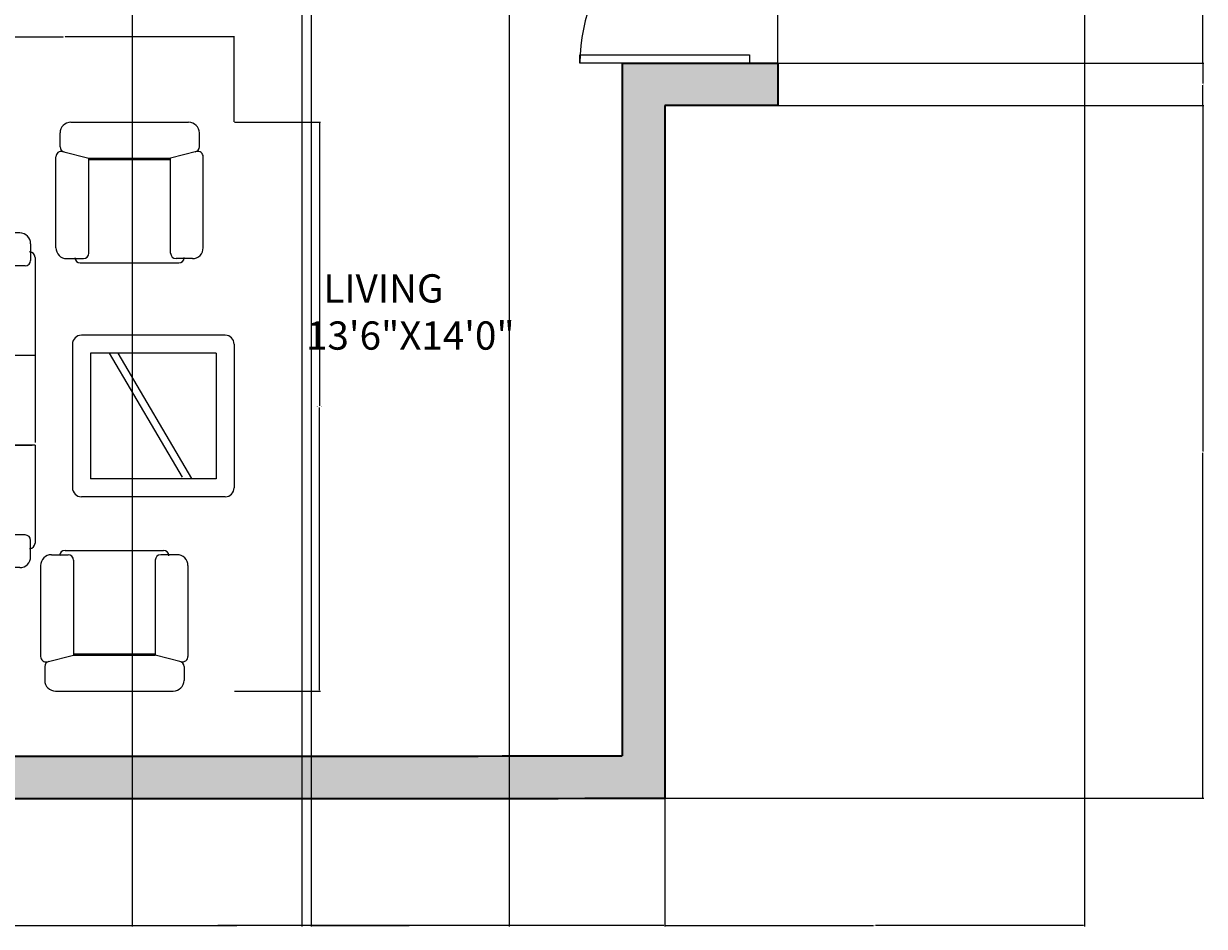
# Model space of a CAD drawing. Units: inches. Extents: x 1044 to 1567, y 918 to 1417.
# Tile 3 of 4: x 1316 to 1567, y 918 to 1110. Entities that reach past the tile are written whole.
import ezdxf

# ---------------------------------------------------------------- set-up
doc = ezdxf.new("R2010")
doc.units = ezdxf.units.IN
for name, color, linetype, lineweight in [('A-ANNO-DIMS', 2, 'Continuous', 18), ('A-AREA-IDEN', 7, 'Continuous', 18), ('A-FLOR', 7, 'Continuous', 13), ('A-FURN', 8, 'Continuous', 18), ('A-WALL', 7, 'Continuous', 35), ('A-WALL-PATT', 252, 'Continuous', 13), ('door', 4, 'Continuous', 18)]:
    doc.layers.add(name, color=color, linetype=linetype, lineweight=lineweight)
doc.styles.get("Standard").update_dxf_attribs({"font": 'arial.ttf'})
doc.dimstyles.get("Standard").update_dxf_attribs({"dimtxt": 0.18, "dimasz": 0.18, "dimexe": 0.18, "dimexo": 0.0625, "dimgap": 0.09, "dimtad": 0, "dimtih": 1, "dimtoh": 1, "dimdec": 4, "dimzin": 0, "dimdsep": 46, "dimtxsty": 'Standard', "dimcen": 0.09, "dimadec": 0, "dimazin": 0, "dimtfac": 1, "dimtdec": 4, "dimtofl": 0, "dimtmove": 0, "dimatfit": 3, "dimfxl": 1, "dimtolj": 1, "dimtzin": 0, "dimarcsym": 0})

# ---------------------------------------------------------------- blocks, each defined once
blk = doc.blocks.new('*U5')
for p, q in [((-36, 0), (-36, 6)), ((0, 0), (0, 6))]:
    blk.add_line(p, q)
blk.add_lwpolyline([(0, 0), (0, -36), (-1.75, -36), (-1.75, 0)], close=True)
blk.add_arc((0, 0), 36, 180, 270)
blk = doc.blocks.new('A$C151D5484')
for p, q in [((1369.5, 1892.5), (769.5, 1892.5)), ((1369, 1877.5), (1369, 1123.6)), ((1369.5, 1108.6), (1369.5, 1892.5)), ((2468.2, 1892.5), (1384, 1892.5)), ((1869.5, 1108.6), (1869.5, 1892.5)), ((709.5, 1762.5), (709.5, 1832.5)), ((2528.2, 1756), (2528.2, 1832.5)), ((709.5, 1756), (709.5, 1762.5)), ((725.3, 1728.6), (869.5, 1692.5)), ((2514.2, 1729), (2368.2, 1692.5)), ((202.4, 1601.7), (169.9, 1679.1)), ((169.9, 1679.1), (199.5, 1598.8)), ((254.6, 1562.3), (213.8, 1708.1)), ((213.8, 1708.1), (254.6, 1560.8)), ((237.9, 1617.5), (261.5, 1673.1)), ((356.6, 1687.9), (254.6, 1562.3)), ((261.5, 1560.8), (356.6, 1687.9)), ((312.8, 1632.7), (315.2, 1673.1)), ((688, 1193.1), (688, 1699.5)), ((869.5, 1163.1), (869.5, 1692.5)), ((1369.5, 1692.5), (869.5, 1692.5)), ((1369.5, 1684.5), (869.5, 1684.5)), ((2368.2, 1692.5), (1384, 1692.5)), ((2368.2, 1684.5), (1384, 1684.5)), ((2368.2, 1163.1), (2368.2, 1692.5)), ((2551.5, 1193.1), (2551.5, 1699.9)), ((199.5, 1598.8), (126.1, 1614.5)), ((126.1, 1614.5), (203.9, 1591.9)), ((254.6, 1560.8), (202.4, 1601.7)), ((203.9, 1591.9), (253.2, 1557.9)), ((253.2, 1557.9), (212.3, 1582.5)), ((212.3, 1582.5), (253.2, 1546.1)), ((316.7, 1566.8), (396, 1625.4)), ((396, 1625.4), (321.1, 1560.8)), ((321.1, 1560.8), (340.3, 1608.6)), ((253.2, 1546.1), (123.1, 1497.8)), ((123.1, 1497.8), (260.1, 1544.6)), ((144.8, 1448.6), (187.2, 1521.4)), ((177.3, 1514.1), (144.8, 1448.6)), ((260.1, 1544.6), (177.3, 1514.1)), ((187.2, 1521.4), (261.5, 1540.2)), ((409.3, 1572.7), (261.5, 1560.8)), ((261.5, 1540.2), (273.4, 1416.5)), ((273.4, 1416.5), (264.5, 1553.5)), ((264.5, 1553.5), (347.2, 1433.8)), ((271.9, 1556.4), (403.4, 1569.7)), ((343.3, 1524.4), (271.9, 1556.4)), ((271.9, 1552), (343.3, 1524.4)), ((347.2, 1433.8), (271.9, 1552)), ((403.4, 1569.7), (316.7, 1566.8)), ((267.9, 1476.6), (221.2, 1427.3)), ((317.2, 1485.5), (360, 1472.6)), ((748, 1133.1), (839.5, 1133.1)), ((2491.5, 1133.1), (2398.2, 1133.1)), ((136.6, 1054.2), (60, 1054.2)), ((699.4, 1077.4), (192.6, 1077.4)), ((1369.5, 1108.6), (823.9, 1108.6)), ((2415.6, 1108.6), (1384, 1108.6)), ((0, 994.2), (0, 338.9)), ((163.5, 1040.2), (200, 894.2)), ((759.4, 1017.4), (759.4, 924.2)), ((2468.8, 992.3), (2975.6, 992.3)), ((783.9, 941.5), (783.9, 393.4)), ((2408.8, 932.3), (2408.8, 839.1)), ((3004.7, 955.1), (2968.2, 809.1)), ((3031.7, 969.1), (3108.2, 969.1)), ((729.4, 894.2), (200, 894.2)), ((200, 894.2), (200, 438.9)), ((208, 894.2), (208, 438.9)), ((1932.2, 900), (1132.2, 900)), ((2384.3, 856.4), (2384.3, 308.3)), ((3168.2, 909.1), (3168.2, 253.8)), ((1082.2, 50), (1082.2, 850)), ((1182.2, 100), (1182.2, 800)), ((1882.2, 800), (1182.2, 800)), ((1882.2, 100), (1882.2, 800)), ((1982.2, 50), (1982.2, 850)), ((2438.8, 809.1), (2968.2, 809.1)), ((2960.2, 809.1), (2960.2, 353.8)), ((2968.2, 809.1), (2968.2, 353.8)), ((1882.2, 695.3), (1190.6, 289.3)), ((1882.2, 647.3), (1183.2, 237)), ((164, 294.7), (200, 438.9)), ((729.4, 438.9), (200, 438.9)), ((759.4, 317.5), (759.4, 408.9)), ((2438.8, 353.8), (2968.2, 353.8)), ((3004.3, 209.6), (2968.2, 353.8)), ((130, 278.9), (60, 278.9)), ((136.6, 278.9), (130, 278.9)), ((2408.8, 232.4), (2408.8, 323.8)), ((699.4, 257.5), (193.1, 257.5)), ((2468.8, 172.4), (2975.2, 172.4)), ((3031.7, 193.8), (3038.2, 193.8)), ((3038.2, 193.8), (3108.2, 193.8)), ((1882.2, 100), (1182.2, 100)), ((1932.2, 0), (1132.2, 0))]:
    blk.add_line(p, q)
for centre, radius, start, end in [((769.5, 1832.5), 60, 90, 180), ((1384, 1877.5), 15, 90, 180), ((2468.2, 1832.5), 60, 0, 90), ((187.1, 1731), 24.5, 161.81925, 230.08176), ((177.5, 1725), 30.6, 324.97446, 61.37923), ((205.1, 1714.3), 38.8, 10.87616, 75.44791), ((232.7, 1706.8), 29.4, 330.50948, 39.29199), ((288.1, 1741.4), 26.5, 134.25765, 198.59266), ((270.3, 1743.8), 33.6, 300.94824, 20.57839), ((354.9, 1734.8), 35.6, 159.72014, 225.64891), ((356.2, 1726.1), 15.5, 253.49335, 4.46973), ((718, 1699.5), 30, 75.96376, 180), ((739.5, 1756), 30, 180, 255.96376), ((2498.2, 1756), 30, 284.03624, 0), ((2521.5, 1699.9), 30, 0, 104.03624), ((101.2, 1661.9), 17.2, 166.54191, 283.47743), ((97.2, 1657.3), 37.3, 1.63276, 82.02679), ((134, 1678.6), 27.3, 23.47529, 113.45596), ((162.1, 1676.6), 26.2, 357.17243, 67.23647), ((352.5, 1680.1), 26.5, 112.57231, 188.33354), ((400.1, 1673.2), 34.4, 93.31893, 173.19037), ((400.2, 1620.3), 23.4, 78.8066, 167.6391), ((385.7, 1677.6), 24.4, 295.45365, 26.6852), ((434, 1633.1), 18.9, 56.81507, 154.01934), ((1384, 1677.5), 15, 90, 180), ((1384, 1669.5), 15, 90, 180), ((87.4, 1616.2), 38, 212.11699, 291.72753), ((92.9, 1593.6), 31.9, 69.11699, 140.36062), ((113.9, 1603.3), 33.6, 32.88731, 96.72533), ((430.1, 1640.4), 35.1, 239.47372, 321.75859), ((464, 1564.4), 34.3, 102.30595, 169.6849), ((71, 1577), 21.9, 219.74751, 296.0709), ((92.8, 1505.2), 29.6, 95.31956, 170.41897), ((104.7, 1572.3), 26.4, 238.78766, 311.59771), ((412, 1579.3), 27.9, 235.52479, 310.83273), ((453.3, 1557.3), 47.8, 223.81169, 284.30773), ((449.1, 1531.3), 22, 35.40933, 112.71009), ((93.9, 1448.7), 51.8, 75.20711, 128.32175), ((94.4, 1445), 22.5, 66.77542, 141.28797), ((143.4, 1427), 33.9, 128.69621, 196.24154), ((117.4, 1490.2), 24.6, 263.64998, 344.65145), ((403.5, 1495.1), 24.1, 193.89139, 288.90395), ((433.5, 1458.5), 49.5, 190.3005, 250.44765), ((406.6, 1435.2), 28.2, 14.10036, 78.46502), ((440.2, 1444.2), 48, 73.46423, 122.79056), ((116.6, 1437.1), 40.7, 276.54869, 346.89113), ((149.8, 1398.4), 17.7, 269.25572, 357.62866), ((204.2, 1410.8), 27.1, 118.80717, 193.91988), ((220.2, 1388.5), 31.6, 161.37117, 231.75354), ((200, 1381.3), 34.2, 299.1952, 16.7189), ((284.5, 1402.5), 27.3, 148.87476, 221.21352), ((306.7, 1385.5), 27.7, 180.25287, 263.52208), ((290.4, 1371.7), 38.6, 334.73526, 50.57812), ((320.2, 1409.1), 27.9, 356.02822, 71.36976), ((340.3, 1378.7), 18.7, 329.98145, 65.66759), ((383.9, 1431.1), 26.9, 212.58173, 297.17999), ((240.9, 1363.2), 18.8, 298.19814, 22.19179), ((748, 1193.1), 60, 180, 270), ((2491.5, 1193.1), 60, 270, 0), ((823.9, 1138.6), 30, 180, 270), ((839.5, 1163.1), 30, 270, 0), ((2398.2, 1163.1), 30, 180, 270), ((2415.6, 1138.6), 30, 270, 0), ((60, 994.2), 60, 90, 180), ((136.6, 1024.2), 30, 14.03624, 90), ((192.6, 1047.4), 30, 90, 194.03624), ((699.4, 1017.4), 60, 0, 90), ((2468.8, 932.3), 60, 90, 180), ((2975.6, 962.3), 30, 345.96376, 90), ((729.4, 924.2), 30, 270, 0), ((753.9, 941.5), 30, 0, 90), ((3031.7, 939.1), 30, 90, 165.96376), ((3108.2, 909.1), 60, 0, 90), ((1132.2, 850), 50, 90, 180), ((1932.2, 850), 50, 0, 90), ((2414.3, 856.4), 30, 90, 180), ((2438.8, 839.1), 30, 180, 270), ((729.4, 408.9), 30, 0, 90), ((60, 338.9), 60, 180, 270), ((753.9, 393.4), 30, 270, 0), ((2438.8, 323.8), 30, 90, 180), ((136.6, 308.9), 30, 270, 345.96376), ((193.1, 287.5), 30, 165.96376, 270), ((699.4, 317.5), 60, 270, 0), ((2414.3, 308.3), 30, 180, 270), ((2468.8, 232.4), 60, 180, 270), ((2975.2, 202.4), 30, 270, 14.03624), ((3031.7, 223.8), 30, 194.03624, 270), ((3108.2, 253.8), 60, 270, 0), ((1132.2, 50), 50, 180, 270), ((1932.2, 50), 50, 270, 0)]:
    blk.add_arc(centre, radius, start, end)
blk = doc.blocks.new('*D22')
at = {"layer": 'A-ANNO-DIMS', "color": 0, "lineweight": -2, "transparency": 16777216}
for p, q in [((1360.9, 1089.11), (1379.13, 1089.11)), ((1378.95, 1088.93), (1378.95, 1028.92)), ((1378.95, 968.55), (1378.95, 1028.56)), ((1360.9, 968.37), (1379.13, 968.37))]:
    blk.add_line(p, q, dxfattribs=at)
at = {"layer": 'A-ANNO-DIMS', "color": 0, "transparency": 16777216}
for points in [[(1378.92, 1088.93), (1378.98, 1088.93), (1378.95, 1089.11)], [(1378.92, 968.55), (1378.98, 968.55), (1378.95, 968.37)]]:
    blk.add_solid(points, dxfattribs=at)
at = {"layer": 'Defpoints', "color": 0, "transparency": 16777216}
for p in [(1360.84, 1089.11), (1378.95, 1089.11), (1360.84, 968.37)]:
    blk.add_point(p, dxfattribs=at)
at = {"layer": 'A-ANNO-DIMS', "color": 0, "transparency": 16777216, "insert": (1378.95, 1028.74), "char_height": 0.18, "attachment_point": 5}
blk.add_mtext('\\A1;LIVING GROUP 121', dxfattribs=at)
blk = doc.blocks.new('*D23')
at = {"layer": 'A-ANNO-DIMS', "color": 0, "lineweight": -2, "transparency": 16777216}
for p, q in [((1288.72, 1089.17), (1288.72, 1107.4)), ((1288.9, 1107.22), (1324.56, 1107.22)), ((1360.66, 1107.22), (1325, 1107.22)), ((1360.84, 1089.17), (1360.84, 1107.4))]:
    blk.add_line(p, q, dxfattribs=at)
at = {"layer": 'A-ANNO-DIMS', "color": 0, "transparency": 16777216}
for points in [[(1288.9, 1107.25), (1288.9, 1107.19), (1288.72, 1107.22)], [(1360.66, 1107.25), (1360.66, 1107.19), (1360.84, 1107.22)]]:
    blk.add_solid(points, dxfattribs=at)
at = {"layer": 'Defpoints', "color": 0, "transparency": 16777216}
for p in [(1288.72, 1107.22), (1288.72, 1089.11), (1360.84, 1089.11)]:
    blk.add_point(p, dxfattribs=at)
at = {"layer": 'A-ANNO-DIMS', "color": 0, "transparency": 16777216, "insert": (1324.78, 1107.22), "char_height": 0.18, "attachment_point": 5}
blk.add_mtext('\\A1;72', dxfattribs=at)
blk = doc.blocks.new('*D34')
at = {"layer": 'A-ANNO-DIMS', "color": 0, "lineweight": -2, "transparency": 16777216}
for p, q in [((1271.18, 945.49), (1271.18, 918.44)), ((1452.18, 945.57), (1452.18, 918.44)), ((1271.36, 918.62), (1361.41, 918.62)), ((1452, 918.62), (1361.94, 918.62))]:
    blk.add_line(p, q, dxfattribs=at)
at = {"layer": 'A-ANNO-DIMS', "color": 0, "transparency": 16777216}
for points in [[(1271.36, 918.65), (1271.36, 918.59), (1271.18, 918.62)], [(1452, 918.65), (1452, 918.59), (1452.18, 918.62)]]:
    blk.add_solid(points, dxfattribs=at)
at = {"layer": 'Defpoints', "color": 0, "transparency": 16777216}
for p in [(1271.18, 945.56), (1452.18, 945.63), (1452.18, 918.62)]:
    blk.add_point(p, dxfattribs=at)
at = {"layer": 'A-ANNO-DIMS', "color": 0, "transparency": 16777216, "insert": (1361.68, 918.62), "char_height": 0.18, "attachment_point": 5}
blk.add_mtext('\\A1;181', dxfattribs=at)
blk = doc.blocks.new('*D35')
at = {"layer": 'A-ANNO-DIMS', "color": 0, "lineweight": -2, "transparency": 16777216}
for p, q in [((1541.18, 1137.7), (1541.18, 918.44)), ((1452.18, 945.57), (1452.18, 918.44)), ((1452.36, 918.62), (1496.46, 918.62)), ((1541, 918.62), (1496.9, 918.62))]:
    blk.add_line(p, q, dxfattribs=at)
at = {"layer": 'A-ANNO-DIMS', "color": 0, "transparency": 16777216}
for points in [[(1452.36, 918.65), (1452.36, 918.59), (1452.18, 918.62)], [(1541, 918.65), (1541, 918.59), (1541.18, 918.62)]]:
    blk.add_solid(points, dxfattribs=at)
at = {"layer": 'Defpoints', "color": 0, "transparency": 16777216}
for p in [(1541.18, 1137.77), (1452.18, 945.63), (1541.18, 918.62)]:
    blk.add_point(p, dxfattribs=at)
at = {"layer": 'A-ANNO-DIMS', "color": 0, "transparency": 16777216, "insert": (1496.68, 918.62), "char_height": 0.18, "attachment_point": 5}
blk.add_mtext('\\A1;89', dxfattribs=at)
blk = doc.blocks.new('*D36')
at = {"layer": 'A-ANNO-DIMS', "color": 0, "lineweight": -2, "transparency": 16777216}
for p, q in [((1452.24, 1092.64), (1566.52, 1092.64)), ((1566.34, 1092.46), (1566.34, 1019.32)), ((1566.34, 945.81), (1566.34, 1018.95)), ((1452.24, 945.63), (1566.52, 945.63))]:
    blk.add_line(p, q, dxfattribs=at)
at = {"layer": 'A-ANNO-DIMS', "color": 0, "transparency": 16777216}
for points in [[(1566.31, 1092.46), (1566.37, 1092.46), (1566.34, 1092.64)], [(1566.31, 945.81), (1566.37, 945.81), (1566.34, 945.63)]]:
    blk.add_solid(points, dxfattribs=at)
at = {"layer": 'Defpoints', "color": 0, "transparency": 16777216}
for p in [(1452.18, 1092.64), (1566.34, 1092.64), (1452.18, 945.63)]:
    blk.add_point(p, dxfattribs=at)
at = {"layer": 'A-ANNO-DIMS', "color": 0, "transparency": 16777216, "insert": (1566.34, 1019.14), "char_height": 0.18, "attachment_point": 5}
blk.add_mtext('\\A1;147', dxfattribs=at)
blk = doc.blocks.new('*D37')
at = {"layer": 'A-ANNO-DIMS', "color": 0, "lineweight": -2, "transparency": 16777216}
for p, q in [((1476.24, 1101.64), (1566.52, 1101.64)), ((1566.34, 1101.46), (1566.34, 1097.32)), ((1566.34, 1092.82), (1566.34, 1096.95)), ((1476.24, 1092.64), (1566.52, 1092.64))]:
    blk.add_line(p, q, dxfattribs=at)
at = {"layer": 'A-ANNO-DIMS', "color": 0, "transparency": 16777216}
for points in [[(1566.31, 1101.46), (1566.37, 1101.46), (1566.34, 1101.64)], [(1566.31, 1092.82), (1566.37, 1092.82), (1566.34, 1092.64)]]:
    blk.add_solid(points, dxfattribs=at)
at = {"layer": 'Defpoints', "color": 0, "transparency": 16777216}
for p in [(1476.18, 1101.64), (1566.34, 1101.64), (1476.18, 1092.64)]:
    blk.add_point(p, dxfattribs=at)
at = {"layer": 'A-ANNO-DIMS', "color": 0, "transparency": 16777216, "insert": (1566.34, 1097.14), "char_height": 0.18, "attachment_point": 5}
blk.add_mtext('\\A1;9', dxfattribs=at)
blk = doc.blocks.new('*D38')
at = {"layer": 'A-ANNO-DIMS', "color": 0, "lineweight": -2, "transparency": 16777216}
for p, q in [((1476.24, 1137.66), (1566.52, 1137.66)), ((1566.34, 1137.48), (1566.34, 1119.83)), ((1566.34, 1101.82), (1566.34, 1119.47)), ((1476.24, 1101.64), (1566.52, 1101.64))]:
    blk.add_line(p, q, dxfattribs=at)
at = {"layer": 'A-ANNO-DIMS', "color": 0, "transparency": 16777216}
for points in [[(1566.31, 1137.48), (1566.37, 1137.48), (1566.34, 1137.66)], [(1566.31, 1101.82), (1566.37, 1101.82), (1566.34, 1101.64)]]:
    blk.add_solid(points, dxfattribs=at)
at = {"layer": 'Defpoints', "color": 0, "transparency": 16777216}
for p in [(1476.18, 1137.66), (1566.34, 1137.66), (1476.18, 1101.64)]:
    blk.add_point(p, dxfattribs=at)
at = {"layer": 'A-ANNO-DIMS', "color": 0, "transparency": 16777216, "insert": (1566.34, 1119.65), "char_height": 0.18, "attachment_point": 5}
blk.add_mtext('\\A1;36.03', dxfattribs=at)
blk = doc.blocks.new('*D58')
at = {"layer": 'A-ANNO-DIMS', "color": 0, "lineweight": -2, "transparency": 16777216}
for p, q in [((1339.18, 1236.49), (1339.18, 918.44)), ((1375.18, 1236.49), (1375.18, 918.44)), ((1339.36, 918.62), (1356.96, 918.62)), ((1375, 918.62), (1357.4, 918.62))]:
    blk.add_line(p, q, dxfattribs=at)
at = {"layer": 'A-ANNO-DIMS', "color": 0, "transparency": 16777216}
for points in [[(1339.36, 918.65), (1339.36, 918.59), (1339.18, 918.62)], [(1375, 918.65), (1375, 918.59), (1375.18, 918.62)]]:
    blk.add_solid(points, dxfattribs=at)
at = {"layer": 'Defpoints', "color": 0, "transparency": 16777216}
for p in [(1339.18, 1236.56), (1375.18, 1236.56), (1375.18, 918.62)]:
    blk.add_point(p, dxfattribs=at)
at = {"layer": 'A-ANNO-DIMS', "color": 0, "transparency": 16777216, "insert": (1357.18, 918.62), "char_height": 0.18, "attachment_point": 5}
blk.add_mtext('\\A1;36', dxfattribs=at)
blk = doc.blocks.new('*D59')
at = {"layer": 'A-ANNO-DIMS', "color": 0, "lineweight": -2, "transparency": 16777216}
for p, q in [((1377.18, 1236.49), (1377.18, 918.44)), ((1419.18, 1236.49), (1419.18, 918.44)), ((1377.36, 918.62), (1397.96, 918.62)), ((1419, 918.62), (1398.4, 918.62))]:
    blk.add_line(p, q, dxfattribs=at)
at = {"layer": 'A-ANNO-DIMS', "color": 0, "transparency": 16777216}
for points in [[(1377.36, 918.65), (1377.36, 918.59), (1377.18, 918.62)], [(1419, 918.65), (1419, 918.59), (1419.18, 918.62)]]:
    blk.add_solid(points, dxfattribs=at)
at = {"layer": 'Defpoints', "color": 0, "transparency": 16777216}
for p in [(1377.18, 1236.56), (1419.18, 1236.56), (1419.18, 918.62)]:
    blk.add_point(p, dxfattribs=at)
at = {"layer": 'A-ANNO-DIMS', "color": 0, "transparency": 16777216, "insert": (1398.18, 918.62), "char_height": 0.18, "attachment_point": 5}
blk.add_mtext('\\A1;42', dxfattribs=at)

msp = doc.modelspace()

# ---------------------------------------------------------------- hatches: boundary and pattern name
at = {"layer": 'A-WALL-PATT'}
h = msp.add_hatch(color=256, dxfattribs=at)
h.dxf.hatch_style = 1
h.paths.add_polyline_path([(1476.177, 1101.635), (1452.177, 1101.635, -0.0000174), (1443.177, 1101.625), (1443.177, 954.625, -0.0003145), (1280.177, 954.554), (1280.177, 1099.554, -0.0001275), (1214.177, 1099.584), (1214.177, 1101.584, -0.0000097), (1209.177, 1101.587), (1209.177, 1061.587, 0.0000097), (1214.177, 1061.584), (1214.177, 1094.584, 0.0001178), (1275.177, 1094.555), (1275.177, 1001.555, -0.0000357), (1256.677, 1001.561), (1256.674, 996.561, 0.000028), (1271.177, 996.556), (1271.177, 969.556, -0.0000087), (1266.677, 969.557), (1266.674, 964.557, 0.0000087), (1271.177, 964.556), (1271.177, 945.556, 0.0003493), (1452.177, 945.635), (1452.177, 1092.635), (1476.177, 1092.635)])

# ---------------------------------------------------------------- linework, layer by layer
at = {"layer": 'A-FLOR'}
msp.add_line((1476.177, 1092.635), (1476.177, 1137.665), dxfattribs=at)
at = {"layer": 'A-WALL'}
for p, q in [((1443.177, 1101.625), (1443.177, 954.625)), ((1452.177, 1101.635), (1476.177, 1101.635)), ((1476.177, 1101.635), (1476.177, 1092.635)), ((1452.177, 1092.635), (1452.177, 945.635)), ((1476.177, 1092.635), (1452.177, 1092.635))]:
    msp.add_line(p, q, dxfattribs=at)
for radius, start, end in [(129406.864, 270.06110046, 270.06508528), (129553.864, 269.98894364, 270.06103113), (129562.864, 269.98496439, 270.06500691)]:
    msp.add_arc((1305.177, 130508.416), radius, start, end, dxfattribs=at)

# ---------------------------------------------------------------- block references
at = {"layer": 'A-FURN', "xscale": 0.0381098975720578, "yscale": 0.0381098975720578, "zscale": 0.0381098975720578, "rotation": 90}
msp.add_blockref('A$C151D5484', (1360.841, 968.371), dxfattribs=at)
at = {"layer": 'door', "rotation": 270}
msp.add_blockref('*U5', (1470.177, 1101.635), dxfattribs=at)

# ---------------------------------------------------------------- texts
at = {"layer": 'A-AREA-IDEN', "insert": (1376.086, 1056.836), "char_height": 6, "attachment_point": 1}
msp.add_mtext_dynamic_manual_height_columns('  LIVING\\P13\'6"X14\'0"', width=56.12489, gutter_width=12.5, heights=[0], dxfattribs=at)

# ---------------------------------------------------------------- dimensions: what is measured, and where the dimension line sits
at = {"layer": 'A-ANNO-DIMS'}
for base, p1, p2, picture, middle in [((1375.177, 918.617), (1339.177, 1236.556), (1375.177, 1236.556), '*D58', (1357.177, 918.617)), ((1419.177, 918.617), (1377.177, 1236.556), (1419.177, 1236.556), '*D59', (1398.177, 918.617)), ((1541.177, 918.617), (1452.177, 945.635), (1541.177, 1137.767), '*D35', (1496.677, 918.617)), ((1452.177, 918.617), (1271.177, 945.556), (1452.177, 945.635), '*D34', (1361.677, 918.617))]:
    dim = msp.add_linear_dim(base=base, p1=p1, p2=p2, dimstyle='Standard', override={"dimdec": 0, "dimlfac": 1, "dimrnd": 0, "dimzin": 0, "dimdsep": 46, "dimlunit": 2}, dxfattribs=at)
    dim.commit()
    dim.dimension.update_dxf_attribs({"geometry": picture, "text_midpoint": middle})
for base, p1, p2, angle, override, picture, middle in [((1566.336, 1137.665), (1476.177, 1101.635), (1476.177, 1137.665), 90, {"dimdec": 2, "dimlfac": 1, "dimrnd": 0, "dimzin": 0, "dimdsep": 46, "dimlunit": 2}, '*D38', (1566.336, 1119.65)), ((1288.717, 1107.224), (1360.841, 1089.112), (1288.717, 1089.112), 180, {"dimdec": 0, "dimlfac": 1, "dimrnd": 0, "dimzin": 0, "dimdsep": 46, "dimlunit": 2}, '*D23', (1324.779, 1107.224)), ((1566.336, 1101.635), (1476.177, 1092.635), (1476.177, 1101.635), 90, {"dimdec": 0, "dimlfac": 1, "dimrnd": 0, "dimzin": 0, "dimdsep": 46, "dimlunit": 2}, '*D37', (1566.336, 1097.135)), ((1566.336, 1092.635), (1452.177, 945.635), (1452.177, 1092.635), 90, {"dimdec": 0, "dimlfac": 1, "dimrnd": 0, "dimzin": 0, "dimdsep": 46, "dimlunit": 2}, '*D36', (1566.336, 1019.135))]:
    dim = msp.add_linear_dim(base=base, p1=p1, p2=p2, angle=angle, dimstyle='Standard', override=override, dxfattribs=at)
    dim.commit()
    dim.dimension.update_dxf_attribs({"geometry": picture, "text_midpoint": middle})
dim = msp.add_linear_dim(base=(1378.952, 1089.112), p1=(1360.841, 968.371), p2=(1360.841, 1089.112), angle=90, text='LIVING GROUP <>', dimstyle='Standard', override={"dimdec": 0, "dimlfac": 1, "dimrnd": 0, "dimzin": 0, "dimdsep": 46, "dimlunit": 2}, dxfattribs=at)
dim.commit()
dim.dimension.update_dxf_attribs({"geometry": '*D22', "text_midpoint": (1378.952, 1028.742)})

doc.saveas('drawing.dxf')
